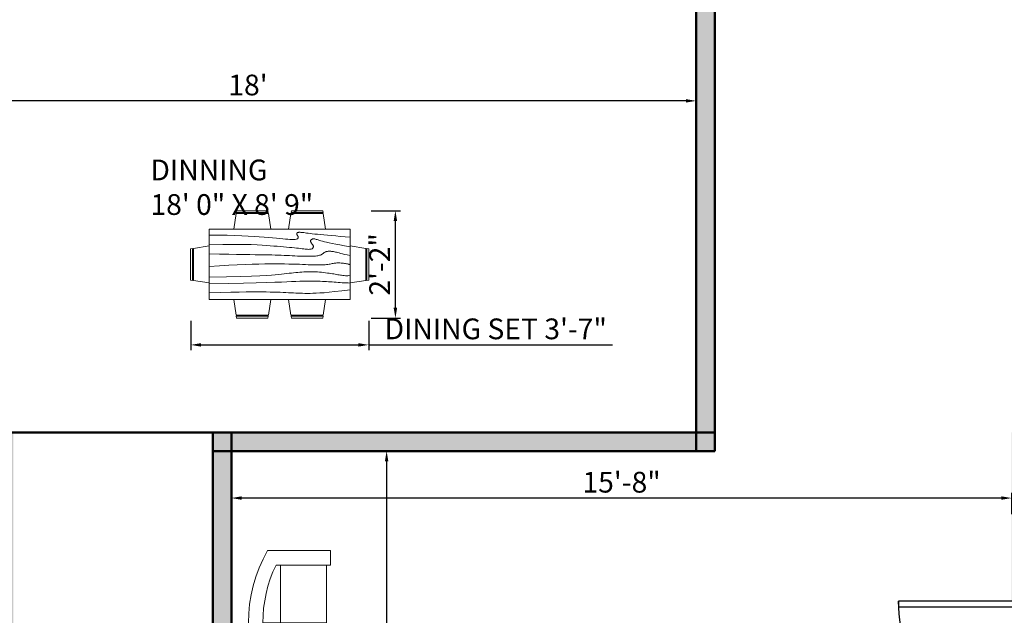
# Model space of a CAD drawing. Units: millimetres. Extents: x 3107 to 3757, y 777 to 1464.
# Tile 5 of 7: x 3301 to 3539, y 1140 to 1284. Entities that reach past the tile are written whole.
import ezdxf

# ---------------------------------------------------------------- set-up
doc = ezdxf.new("R2010")
doc.units = ezdxf.units.MM
for name, color, linetype, lineweight in [('A-ANNO-DIMS', 50, 'Continuous', 18), ('A-AREA-IDEN', 160, 'Continuous', 18), ('A-WALL-PATT', 80, 'Continuous', 13), ('doors', 10, 'Continuous', 25), ('furniture', 140, 'Continuous', 18), ('walls', 80, 'Continuous', 50)]:
    doc.layers.add(name, color=color, linetype=linetype, lineweight=lineweight)
doc.styles.get("Standard").update_dxf_attribs({"font": 'arial.ttf'})
doc.dimstyles.new('ISO-25', dxfattribs={"dimtxt": 5, "dimasz": 2.5, "dimexe": 1.25, "dimexo": 0.625, "dimtad": 1, "dimdec": 0, "dimlunit": 3, "dimtxsty": 'Standard', "dimcen": 2.5, "dimadec": 0, "dimazin": 0, "dimtfac": 1, "dimtdec": 0, "dimtmove": 0, "dimatfit": 3, "dimfxl": 1, "dimarcsym": 0})

# ---------------------------------------------------------------- blocks, each defined once
blk = doc.blocks.new('*U2')
for p, q in [((0, 0), (0, -6)), ((40, 0), (40, -6))]:
    blk.add_line(p, q)
blk.add_lwpolyline([(0, 0), (0, 40), (1.75, 40), (1.75, 0)], close=True)
blk.add_arc((0, 0), 40, 0, 90)
blk = doc.blocks.new('Dining Set - 36 x 72 in.')
for p, q in [((-22.2343, 26.00059), (-23.4847, 17.99762)), ((-22.2304, 26), (-5.7608, 26)), ((-22, 27.5), (-22.1562, 26.50042)), ((-5.8416, 26.5), (-22.1534, 26.5)), ((-22, 27.5), (-6, 27.5)), ((-5.8437, 26.49966), (-6, 27.5)), ((-4.5152, 17.99762), (-5.7655, 25.99926)), ((5.7657, 26.00059), (4.5153, 17.99762)), ((5.7696, 26), (22.2392, 26)), ((6, 27.5), (5.8438, 26.50042)), ((22.1584, 26.5), (5.8466, 26.5)), ((6, 27.5), (22, 27.5)), ((22.1563, 26.49966), (22, 27.5)), ((23.4848, 17.99762), (22.2345, 25.99926)), ((36, 18), (-36, 18)), ((-36, 18), (-36, -18)), ((36, -18), (36, 18)), ((-45.5, 8), (-44.5004, 8.15617)), ((-45.5, 8), (-45.5, -8)), ((-44.5, -8.15843), (-44.5, 8.15338)), ((-44.0006, 8.23428), (-35.9976, 9.48474)), ((-44, 8.23041), (-44, -8.23915)), ((44.0006, 8.23428), (35.9976, 9.48474)), ((44, 8.23041), (44, -8.23915)), ((44.5, -8.15843), (44.5, 8.15338)), ((45.5, 8), (44.5005, 8.15617)), ((45.5, 8), (45.5, -8)), ((-44.4997, -8.15631), (-45.5, -8)), ((-35.9976, -9.48476), (-43.9993, -8.2345)), ((35.9976, -9.48476), (43.9993, -8.2345)), ((44.4997, -8.15631), (45.5, -8)), ((-36, -18), (36, -18)), ((-22.2343, -26.0006), (-23.4847, -17.99762)), ((-4.5152, -17.99762), (-5.7655, -25.99928)), ((5.7657, -26.0006), (4.5153, -17.99762)), ((23.4848, -17.99762), (22.2345, -25.99928)), ((-22.2304, -26), (-5.7608, -26)), ((-22, -27.5), (-22.1562, -26.50044)), ((-5.8416, -26.5), (-22.1534, -26.5)), ((-22, -27.5), (-6, -27.5)), ((-5.8437, -26.49967), (-6, -27.5)), ((5.7696, -26), (22.2392, -26)), ((6, -27.5), (5.8438, -26.50044)), ((22.1584, -26.5), (5.8466, -26.5)), ((6, -27.5), (22, -27.5)), ((22.1563, -26.49967), (22, -27.5))]:
    blk.add_line(p, q)
for points in [[(-36, 15), (-31.1772, 14.97754), (-26.8079, 14.91406), (-22.8538, 14.81543), (-19.276, 14.6875), (-16.0362, 14.53613), (-13.0957, 14.36718), (-10.4159, 14.18652), (-7.9583, 14), (-5.6904, 13.81315), (-3.6035, 13.63021), (-1.6954, 13.45508), (0.0365, 13.29166), (1.5945, 13.14388), (2.9811, 13.01562), (4.1988, 12.9108), (5.25, 12.83333), (6.1393, 12.78613), (6.8802, 12.76823), (7.4883, 12.77767), (7.9792, 12.8125), (8.3685, 12.87077), (8.6719, 12.95052), (8.9049, 13.0498), (9.0833, 13.16666), (9.2205, 13.29899), (9.3216, 13.44401), (9.3895, 13.59879), (9.4271, 13.76041), (9.4373, 13.92594), (9.4232, 14.09245), (9.3875, 14.257), (9.3333, 14.41666), (9.2638, 14.56917), (9.1836, 14.71484), (9.0975, 14.85465), (9.0104, 14.98958), (8.9272, 15.1206), (8.8529, 15.2487), (8.7922, 15.37483), (8.75, 15.5), (8.7305, 15.62467), (8.7344, 15.74739), (8.7617, 15.86621), (8.8125, 15.97916), (8.8867, 16.08431), (8.9844, 16.17968), (9.1055, 16.26334), (9.25, 16.33333), (9.4189, 16.38802), (9.6172, 16.42708), (9.8506, 16.45052), (10.125, 16.45833), (10.4463, 16.45052), (10.8203, 16.42708), (11.2529, 16.38802), (11.75, 16.33333), (12.3184, 16.26318), (12.9694, 16.17838), (13.7151, 16.07991), (14.5677, 15.96875), (15.5395, 15.84586), (16.6426, 15.71224), (17.8893, 15.56884), (19.2917, 15.41666), (20.859, 15.25667), (22.5879, 15.08984), (24.4721, 14.91715), (26.5052, 14.73958), (28.6809, 14.5581), (30.9929, 14.3737), (33.4347, 14.18733), (36, 14)], [(-36, 10), (-28.9766, 10.14274), (-23.1725, 10.20442), (-18.4241, 10.19775), (-14.5677, 10.13541), (-11.4399, 10.03011), (-8.877, 9.89453), (-6.7154, 9.74137), (-4.7917, 9.58333), (-2.9698, 9.43082), (-1.2246, 9.28515), (0.4415, 9.14534), (2.026, 9.01041), (3.5266, 8.87939), (4.9408, 8.7513), (6.266, 8.62516), (7.5, 8.5), (8.6411, 8.37549), (9.6914, 8.2539), (10.6538, 8.13818), (11.5312, 8.03125), (12.3267, 7.93603), (13.043, 7.85547), (13.6831, 7.79248), (14.25, 7.75), (14.7471, 7.7303), (15.1797, 7.73307), (15.5537, 7.75732), (15.875, 7.80208), (16.1494, 7.86637), (16.3828, 7.94922), (16.5811, 8.04964), (16.75, 8.16666), (16.8944, 8.29915), (17.0143, 8.44531), (17.1089, 8.60319), (17.1771, 8.77083), (17.218, 8.94629), (17.2305, 9.1276), (17.2137, 9.31282), (17.1667, 9.5), (17.0895, 9.6875), (16.987, 9.875), (16.8649, 10.0625), (16.7292, 10.25), (16.5856, 10.4375), (16.4401, 10.625), (16.2985, 10.8125), (16.1667, 11), (16.05, 11.18733), (15.9518, 11.3737), (15.8752, 11.5581), (15.8229, 11.73958), (15.798, 11.91715), (15.8034, 12.08984), (15.842, 12.25667), (15.9167, 12.41666), (16.0295, 12.56836), (16.1784, 12.70833), (16.3605, 12.83268), (16.5729, 12.9375), (16.8127, 13.01888), (17.0768, 13.07291), (17.3625, 13.0957), (17.6667, 13.08333), (17.9894, 13.03312), (18.3418, 12.94726), (18.7382, 12.82918), (19.1927, 12.68229), (19.7195, 12.51001), (20.3327, 12.31575), (21.0465, 12.10294), (21.875, 11.875), (22.8357, 11.63354), (23.959, 11.37304), (25.2786, 11.08618), (26.8282, 10.76562), (28.6414, 10.40405), (30.752, 9.99414), (33.1936, 9.52856), (36, 9)], [(-36, 5.5), (-30.7157, 5.3348), (-26.069, 5.20963), (-21.9946, 5.11767), (-18.4271, 5.05208), (-15.3009, 5.00602), (-12.5508, 4.97265), (-10.1112, 4.94515), (-7.9167, 4.91666), (-5.909, 4.88167), (-4.0586, 4.83984), (-2.3429, 4.79215), (-0.7396, 4.73958), (0.7739, 4.6831), (2.22, 4.6237), (3.6213, 4.56233), (5, 4.5), (6.373, 4.43782), (7.7344, 4.3776), (9.0723, 4.32129), (10.375, 4.27083), (11.6309, 4.22819), (12.8281, 4.19531), (13.9551, 4.17415), (15, 4.16666), (15.954, 4.17448), (16.819, 4.19791), (17.6001, 4.23698), (18.3021, 4.29166), (18.9299, 4.36198), (19.4883, 4.44791), (19.9823, 4.54948), (20.4167, 4.66666), (20.7969, 4.79899), (21.1302, 4.94401), (21.4245, 5.09879), (21.6875, 5.26041), (21.9271, 5.42594), (22.1511, 5.59245), (22.3672, 5.757), (22.5834, 5.91666), (22.8065, 6.06868), (23.0404, 6.21093), (23.2879, 6.34147), (23.5521, 6.45833), (23.8358, 6.55957), (24.142, 6.64323), (24.4735, 6.70735), (24.8334, 6.75), (25.2235, 6.76969), (25.642, 6.76692), (26.0858, 6.74267), (26.5521, 6.69791), (27.0379, 6.63362), (27.5404, 6.55078), (28.0565, 6.45036), (28.5834, 6.33333), (29.1242, 6.19987), (29.7071, 6.04687), (30.3661, 5.87044), (31.1354, 5.66666), (32.0493, 5.43164), (33.142, 5.16146), (34.4475, 4.85221), (36, 4.5)], [(-36, -1), (-30.7915, -0.6591), (-26.0195, -0.38216), (-21.6519, -0.16284), (-17.6563, 0.00521), (-14.0005, 0.12833), (-10.6523, 0.21289), (-7.5796, 0.26522), (-4.75, 0.29166), (-2.134, 0.29793), (0.2878, 0.28711), (2.5317, 0.26163), (4.6146, 0.22396), (6.5529, 0.17651), (8.3633, 0.12174), (10.0623, 0.06209), (11.6667, 0), (13.1899, -0.06201), (14.6341, -0.1211), (15.9982, -0.17432), (17.2813, -0.21875), (18.4823, -0.25147), (19.6003, -0.26953), (20.6343, -0.27002), (21.5834, -0.25), (22.4481, -0.20768), (23.2357, -0.14584), (23.9549, -0.06836), (24.6146, 0.02083), (25.2235, 0.11784), (25.7904, 0.21875), (26.3241, 0.31966), (26.8334, 0.41666), (27.3265, 0.50618), (27.8099, 0.58593), (28.2894, 0.65397), (28.7709, 0.70833), (29.2601, 0.74707), (29.763, 0.76823), (30.2855, 0.76985), (30.8334, 0.75), (31.4088, 0.70784), (31.9994, 0.64713), (32.589, 0.57275), (33.1615, 0.48958), (33.7008, 0.4025), (34.1908, 0.3164), (34.6153, 0.23616), (34.9584, 0.16666), (35.2099, 0.11165), (35.3848, 0.07031), (35.504, 0.04069), (35.5886, 0.02083), (35.6594, 0.00879), (35.7377, 0.0026), (35.8442, 0.00032), (36, 0)], [(-36, -6.5), (-27.1843, -6.31267), (-20.084, -6.1263), (-14.469, -5.9419), (-10.1094, -5.76042), (-6.7752, -5.58285), (-4.2363, -5.41016), (-2.2629, -5.24333), (-0.625, -5.08334), (0.8708, -4.93099), (2.2715, -4.78646), (3.5872, -4.64974), (4.8281, -4.52084), (6.0046, -4.39974), (7.127, -4.28646), (8.2053, -4.18099), (9.25, -4.08334), (10.2705, -3.99382), (11.2734, -3.91407), (12.2647, -3.84603), (13.25, -3.79167), (14.2354, -3.75293), (15.2266, -3.73177), (16.2295, -3.73015), (17.25, -3.75), (18.2912, -3.79248), (19.3451, -3.85547), (20.4009, -3.93604), (21.4479, -4.03125), (22.4754, -4.13819), (23.4727, -4.25391), (24.4289, -4.37549), (25.3334, -4.5), (26.1785, -4.62492), (26.9694, -4.74935), (27.7145, -4.87281), (28.4219, -4.99479), (29.1, -5.11483), (29.7572, -5.23242), (30.4016, -5.34709), (31.0417, -5.45834), (31.6837, -5.56437), (32.3262, -5.65821), (32.9658, -5.73153), (33.599, -5.77604), (34.2224, -5.78345), (34.8327, -5.74545), (35.4264, -5.65373), (36, -5.5)], [(-36, -10), (-26.4022, -9.81299), (-18.4675, -9.62891), (-11.9839, -9.45069), (-6.7396, -9.28125), (-2.5226, -9.12354), (0.8789, -8.98047), (3.6769, -8.85498), (6.0833, -8.75), (8.2767, -8.66765), (10.3021, -8.60677), (12.1712, -8.56543), (13.8958, -8.54167), (15.4876, -8.53353), (16.9583, -8.53907), (18.3197, -8.55632), (19.5834, -8.58334), (20.7616, -8.61841), (21.8685, -8.66081), (22.9188, -8.71004), (23.9271, -8.76563), (24.9081, -8.82707), (25.8763, -8.89388), (26.8465, -8.96558), (27.8334, -9.04167), (28.8474, -9.12118), (29.8828, -9.20117), (30.93, -9.27824), (31.9792, -9.34896), (33.0205, -9.40991), (34.0443, -9.45768), (35.0407, -9.48885), (36, -9.5)], [(-36, -14.5), (-30.0881, -14.33513), (-25.0332, -14.21224), (-20.7312, -14.12647), (-17.0781, -14.07292), (-13.97, -14.04671), (-11.3027, -14.04297), (-8.9724, -14.05681), (-6.875, -14.08334), (-4.9224, -14.11833), (-3.0905, -14.16016), (-1.3709, -14.20785), (0.2448, -14.26042), (1.7647, -14.3169), (3.1973, -14.3763), (4.5507, -14.43767), (5.8333, -14.5), (7.0554, -14.5621), (8.235, -14.62175), (9.3922, -14.67652), (10.5469, -14.72396), (11.7192, -14.76164), (12.929, -14.78711), (14.1965, -14.79794), (15.5417, -14.79167), (16.9933, -14.76424), (18.6152, -14.70508), (20.4804, -14.60197), (22.6615, -14.44271), (25.2312, -14.21509), (28.2624, -13.9069), (31.8277, -13.50594), (36, -13)]]:
    blk.add_lwpolyline(points)
blk = doc.blocks.new('Sofa - Roundback Loveseat 5 ft.')
for p, q in [((0, -32.44198), (0, -5.99998)), ((-24, -33.99998), (-24, -11.46958)), ((24.00004, -33.99998), (24.00004, -11.46958)), ((-23.9998, -13.38178), (23.99986, -13.38178)), ((-24, -32.44198), (24.00004, -32.44198))]:
    blk.add_line(p, q)
for points in [[(-24, -33.99998), (-30, -33.99998), (-30, -7.99998)], [(30.00004, -7.99998), (30.00004, -33.99998), (24.00004, -33.99998)]]:
    blk.add_lwpolyline(points)
for centre, radius, start, end in [((0, -60.24998), 60.24998, 60.13715, 119.8628), ((0, -61.38438), 55.38444, 64.32083, 115.6792)]:
    blk.add_arc(centre, radius, start, end)
blk = doc.blocks.new('*D24')
at = {"layer": 'A-ANNO-DIMS', "color": 0, "lineweight": -2, "transparency": 16777216}
for p, q in [((3248.47, 1264.98), (3248.47, 1265.6)), ((3461.97, 1264.35), (3250.97, 1264.35)), ((3464.47, 1264.98), (3464.47, 1265.6))]:
    blk.add_line(p, q, dxfattribs=at)
at = {"layer": 'A-ANNO-DIMS', "color": 0, "transparency": 16777216}
for points in [[(3250.97, 1264.77), (3250.97, 1263.94), (3248.47, 1264.35)], [(3461.97, 1264.77), (3461.97, 1263.94), (3464.47, 1264.35)]]:
    blk.add_solid(points, dxfattribs=at)
at = {"layer": 'Defpoints', "color": 0, "transparency": 16777216}
for p in [(3248.47, 1264.35), (3248.47, 1264.35), (3464.47, 1264.35)]:
    blk.add_point(p, dxfattribs=at)
at = {"layer": 'A-ANNO-DIMS', "color": 0, "transparency": 16777216, "insert": (3356.47, 1267.53), "char_height": 5, "attachment_point": 5}
blk.add_mtext("18'", dxfattribs=at)
blk = doc.blocks.new('*D40')
at = {"layer": 'A-ANNO-DIMS', "color": 0, "lineweight": -2, "transparency": 16777216}
for p, q in [((3385.8, 1179.93), (3391.12, 1179.93)), ((3389.87, 1177.43), (3389.87, 1030.43)), ((3384.41, 1027.93), (3391.12, 1027.93))]:
    blk.add_line(p, q, dxfattribs=at)
at = {"layer": 'A-ANNO-DIMS', "color": 0, "transparency": 16777216}
for points in [[(3389.45, 1177.43), (3390.29, 1177.43), (3389.87, 1179.93)], [(3389.45, 1030.43), (3390.29, 1030.43), (3389.87, 1027.93)]]:
    blk.add_solid(points, dxfattribs=at)
at = {"layer": 'Defpoints', "color": 0, "transparency": 16777216}
for p in [(3385.18, 1179.93), (3383.78, 1027.93), (3389.87, 1027.93)]:
    blk.add_point(p, dxfattribs=at)
at = {"layer": 'A-ANNO-DIMS', "color": 0, "transparency": 16777216, "insert": (3386.69, 1103.93), "char_height": 5, "attachment_point": 5, "rotation": 90}
blk.add_mtext('12\'-8"', dxfattribs=at)
blk = doc.blocks.new('*D41')
at = {"layer": 'A-ANNO-DIMS', "color": 0, "lineweight": -2, "transparency": 16777216}
for p, q in [((3352.47, 1164.68), (3352.47, 1169.84)), ((3540.47, 1164.68), (3540.47, 1169.84)), ((3537.97, 1168.59), (3354.97, 1168.59))]:
    blk.add_line(p, q, dxfattribs=at)
at = {"layer": 'A-ANNO-DIMS', "color": 0, "transparency": 16777216}
for points in [[(3354.97, 1169), (3354.97, 1168.17), (3352.47, 1168.59)], [(3537.97, 1169), (3537.97, 1168.17), (3540.47, 1168.59)]]:
    blk.add_solid(points, dxfattribs=at)
at = {"layer": 'Defpoints', "color": 0, "transparency": 16777216}
for p in [(3352.47, 1168.59), (3352.47, 1164.06), (3540.47, 1164.06)]:
    blk.add_point(p, dxfattribs=at)
at = {"layer": 'A-ANNO-DIMS', "color": 0, "transparency": 16777216, "insert": (3446.47, 1171.76), "char_height": 5, "attachment_point": 5}
blk.add_mtext('15\'-8"', dxfattribs=at)
blk = doc.blocks.new('*D65')
at = {"layer": 'A-ANNO-DIMS', "color": 0, "lineweight": -2, "transparency": 16777216}
for p, q in [((3342.67, 1211.32), (3342.67, 1204.27)), ((3385.56, 1211.32), (3385.56, 1204.27)), ((3345.17, 1205.52), (3383.06, 1205.52)), ((3385.56, 1205.52), (3444.26, 1205.52))]:
    blk.add_line(p, q, dxfattribs=at)
at = {"layer": 'A-ANNO-DIMS', "color": 0, "transparency": 16777216}
for points in [[(3345.17, 1205.93), (3345.17, 1205.1), (3342.67, 1205.52)], [(3383.06, 1205.93), (3383.06, 1205.1), (3385.56, 1205.52)]]:
    blk.add_solid(points, dxfattribs=at)
at = {"layer": 'Defpoints', "color": 0, "transparency": 16777216}
for p in [(3342.67, 1211.95), (3385.56, 1211.95), (3385.56, 1205.52)]:
    blk.add_point(p, dxfattribs=at)
at = {"layer": 'A-ANNO-DIMS', "color": 0, "transparency": 16777216, "insert": (3416.16, 1208.73), "char_height": 5, "attachment_point": 5}
blk.add_mtext('DINING SET 3\'-7"', dxfattribs=at)
blk = doc.blocks.new('*D66')
at = {"layer": 'A-ANNO-DIMS', "color": 0, "lineweight": -2, "transparency": 16777216}
for p, q in [((3386.18, 1237.87), (3393.24, 1237.87)), ((3391.99, 1214.45), (3391.99, 1235.37)), ((3386.18, 1211.95), (3393.24, 1211.95))]:
    blk.add_line(p, q, dxfattribs=at)
at = {"layer": 'A-ANNO-DIMS', "color": 0, "transparency": 16777216}
for points in [[(3391.57, 1235.37), (3392.41, 1235.37), (3391.99, 1237.87)], [(3391.57, 1214.45), (3392.41, 1214.45), (3391.99, 1211.95)]]:
    blk.add_solid(points, dxfattribs=at)
at = {"layer": 'Defpoints', "color": 0, "transparency": 16777216}
for p in [(3385.56, 1237.87), (3391.99, 1237.87), (3385.56, 1211.95)]:
    blk.add_point(p, dxfattribs=at)
at = {"layer": 'A-ANNO-DIMS', "color": 0, "transparency": 16777216, "insert": (3388.85, 1224.91), "char_height": 5, "attachment_point": 5, "rotation": 90}
blk.add_mtext('2\'-2"', dxfattribs=at)

msp = doc.modelspace()

# ---------------------------------------------------------------- hatches: boundary and pattern name
at = {"layer": 'A-WALL-PATT'}
h = msp.add_hatch(color=256, dxfattribs=at)
h.dxf.hatch_style = 1
h.paths.add_polyline_path([(3119.47, 1087.39), (3110.47, 1087.39), (3110.47, 1027.93), (3119.47, 1027.93)])
h.paths.add_polyline_path([(3119.47, 1027.93), (3110.47, 1027.93), (3110.47, 1023.43), (3119.47, 1023.43)])
h.paths.add_polyline_path([(3267.47, 1027.93), (3119.47, 1027.93), (3119.47, 1023.43), (3267.47, 1023.43)])
h.paths.add_polyline_path([(3119.47, 1023.43), (3110.47, 1023.43), (3110.47, 979.44), (3119.47, 979.44)])
h.paths.add_polyline_path([(3299.97, 1179.93), (3295.47, 1179.93), (3295.47, 1027.93), (3299.97, 1027.93)])
h.paths.add_polyline_path([(3295.47, 1027.93), (3271.97, 1027.93), (3271.97, 1023.43), (3295.47, 1023.43)])
h.paths.add_polyline_path([(3271.97, 1027.93), (3267.47, 1027.93), (3267.47, 1023.43), (3271.97, 1023.43)])
h.paths.add_polyline_path([(3299.97, 1027.93), (3295.47, 1027.93), (3295.47, 1023.43), (3299.97, 1023.43)])
h.paths.add_polyline_path([(3299.97, 1184.43), (3295.47, 1184.43), (3295.47, 1179.93), (3299.97, 1179.93)])
h.paths.add_polyline_path([(3295.47, 1184.43), (3288.38, 1184.43), (3288.38, 1182.47), (3288.38, 1179.93), (3295.47, 1179.93)])
h.paths.add_polyline_path([(3352.47, 1179.93), (3347.97, 1179.93), (3347.97, 1027.93), (3352.47, 1027.93)])
h.paths.add_polyline_path([(3352.47, 1184.43), (3347.97, 1184.43), (3347.97, 1179.93), (3352.47, 1179.93)])
h.paths.add_polyline_path([(3464.47, 1184.43), (3352.47, 1184.43), (3352.47, 1179.93), (3464.47, 1179.93)])
h.paths.add_polyline_path([(3468.97, 1288.93), (3464.47, 1288.93), (3464.47, 1184.43), (3468.97, 1184.43)])
h.paths.add_polyline_path([(3468.97, 1184.43), (3464.47, 1184.43), (3464.47, 1179.93), (3468.97, 1179.93)])
h.paths.add_polyline_path([(3195.97, 1248.43), (3191.47, 1248.43), (3191.47, 1184.43), (3195.97, 1184.43)])
h.paths.add_polyline_path([(3195.97, 1184.43), (3191.47, 1184.43), (3191.47, 1179.93), (3195.97, 1179.93)])
h.paths.add_polyline_path([(3191.47, 1184.43), (3183.28, 1184.43), (3183.28, 1181.58), (3183.28, 1179.93), (3191.47, 1179.93)])
h.paths.add_polyline_path([(3243.97, 1184.43), (3195.97, 1184.43), (3195.97, 1179.93), (3243.97, 1179.93)])
h.paths.add_polyline_path([(3257.91, 1182.47), (3257.91, 1184.43), (3248.47, 1184.43), (3248.47, 1179.93), (3258.02, 1179.93, -0.020891)])
h.paths.add_polyline_path([(3248.47, 1184.43), (3243.97, 1184.43), (3243.97, 1179.93), (3248.47, 1179.93)])
h.paths.add_polyline_path([(3248.47, 1189.24), (3247.51, 1189.24), (3243.97, 1189.24), (3243.97, 1184.43), (3248.47, 1184.43)])
h.paths.add_polyline_path([(3166.87, 1184.43), (3119.47, 1184.43), (3119.47, 1179.93), (3166.63, 1179.93), (3166.63, 1181.58, -0.042981)])
h.paths.add_polyline_path([(3119.47, 1184.43), (3110.47, 1184.43), (3110.47, 1179.93), (3119.47, 1179.93)])
h.paths.add_polyline_path([(3119.47, 1248.43), (3110.47, 1248.43), (3110.47, 1184.43), (3119.47, 1184.43)])
h.paths.add_polyline_path([(3119.47, 1179.93), (3110.47, 1179.93), (3110.47, 1140.65), (3119.47, 1140.65)])
h.paths.add_polyline_path([(3119.47, 1288.93), (3110.47, 1288.93), (3110.47, 1252.93), (3119.47, 1252.93)])
h.paths.add_polyline_path([(3119.47, 1252.93), (3110.47, 1252.93), (3110.47, 1248.43), (3119.47, 1248.43)])
h.paths.add_polyline_path([(3191.47, 1252.93), (3119.47, 1252.93), (3119.47, 1248.43), (3191.47, 1248.43)])
h.paths.add_polyline_path([(3195.97, 1288.93), (3191.47, 1288.93), (3191.47, 1252.93), (3195.97, 1252.93)])
h.paths.add_polyline_path([(3195.97, 1252.93), (3191.47, 1252.93), (3191.47, 1248.43), (3195.97, 1248.43)])
h.paths.add_polyline_path([(3248.47, 1293.43), (3243.97, 1293.43), (3243.97, 1288.93), (3248.47, 1288.93)])
h.paths.add_polyline_path([(3243.97, 1293.43), (3195.97, 1293.43), (3195.97, 1288.93), (3243.97, 1288.93)])
h.paths.add_polyline_path([(3303.47, 1293.43), (3248.47, 1293.43), (3248.47, 1288.93), (3303.47, 1288.93)])
h.paths.add_polyline_path([(3248.47, 1288.93), (3243.97, 1288.93), (3243.97, 1205.51, -0.053712), (3247.51, 1205.89), (3248.47, 1205.89)])
h.paths.add_polyline_path([(3191.47, 1293.43), (3119.47, 1293.43), (3119.47, 1288.93), (3191.47, 1288.93)])
h.paths.add_polyline_path([(3119.47, 1293.43), (3110.47, 1293.43), (3110.47, 1288.93), (3119.47, 1288.93)])
h.paths.add_polyline_path([(3119.47, 1322.96, -0.065064), (3111.64, 1321.93), (3110.47, 1321.93), (3110.47, 1293.43), (3119.47, 1293.43)])
h.paths.add_polyline_path([(3195.97, 1293.43), (3191.47, 1293.43), (3191.47, 1288.93), (3195.97, 1288.93)])
h.paths.add_polyline_path([(3119.47, 1450.43), (3110.47, 1450.43), (3110.47, 1441.43), (3119.47, 1441.43)])
h.paths.add_polyline_path([(3119.47, 1441.43), (3110.47, 1441.43), (3110.47, 1352.4), (3111.64, 1352.4), (3119.47, 1352.4)])
h.paths.add_polyline_path([(3176.58, 1450.43), (3119.47, 1450.43), (3119.47, 1441.43), (3176.58, 1441.43)])
h.paths.add_polyline_path([(3323.19, 1450.43), (3307.97, 1450.43), (3307.97, 1441.43), (3323.19, 1441.43)])
h.paths.add_polyline_path([(3307.97, 1450.43), (3303.47, 1450.43), (3303.47, 1441.43), (3307.97, 1441.43)])
h.paths.add_polyline_path([(3303.47, 1450.43), (3229.4, 1450.43), (3229.4, 1441.43), (3303.47, 1441.43)])
h.paths.add_polyline_path([(3307.97, 1441.43), (3303.47, 1441.43), (3303.47, 1363.43), (3307.97, 1363.43)])
h.paths.add_polyline_path([(3307.97, 1363.43), (3303.47, 1363.43), (3303.47, 1358.93), (3307.97, 1358.93)])
h.paths.add_polyline_path([(3307.97, 1358.93), (3303.47, 1358.93), (3303.47, 1342.3), (3305.5, 1342.3, -0.037178), (3307.97, 1342.12)])
h.paths.add_polyline_path([(3379.97, 1363.43), (3307.97, 1363.43), (3307.97, 1358.93), (3379.97, 1358.93)])
h.paths.add_polyline_path([(3384.47, 1393.61), (3383.04, 1393.61), (3379.97, 1393.61), (3379.97, 1363.43), (3384.47, 1363.43)])
h.paths.add_polyline_path([(3384.47, 1363.43), (3379.97, 1363.43), (3379.97, 1358.93), (3384.47, 1358.93)])
h.paths.add_polyline_path([(3384.47, 1358.93), (3379.97, 1358.93), (3379.97, 1293.43), (3384.47, 1293.43)])
h.paths.add_polyline_path([(3384.47, 1441.43), (3379.97, 1441.43), (3379.97, 1409.98, -0.046389), (3383.04, 1410.27), (3384.47, 1410.27)])
h.paths.add_polyline_path([(3384.47, 1450.43), (3379.97, 1450.43), (3379.97, 1441.43), (3384.47, 1441.43)])
h.paths.add_polyline_path([(3379.97, 1450.43), (3357.18, 1450.43), (3357.18, 1441.43), (3379.97, 1441.43)])
h.paths.add_polyline_path([(3432.79, 1450.43), (3384.47, 1450.43), (3384.47, 1441.43), (3432.79, 1441.43)])
h.paths.add_polyline_path([(3540.47, 1450.43), (3484.18, 1450.43), (3484.18, 1441.43), (3540.47, 1441.43)])
h.paths.add_polyline_path([(3544.97, 1450.43), (3540.47, 1450.43), (3540.47, 1441.43), (3544.97, 1441.43)])
h.paths.add_polyline_path([(3544.97, 1441.43), (3540.47, 1441.43), (3540.47, 1293.43), (3544.97, 1293.43)])
h.paths.add_polyline_path([(3590.83, 1450.43), (3544.97, 1450.43), (3544.97, 1441.43), (3590.83, 1441.43)])
h.paths.add_polyline_path([(3712.97, 1450.43), (3645.62, 1450.43), (3645.62, 1441.43), (3712.97, 1441.43)])
h.paths.add_polyline_path([(3721.97, 1441.43), (3712.97, 1441.43), (3712.97, 1288.93), (3712.97, 1184.43), (3721.97, 1184.43), (3721.97, 1288.93)])
h.paths.add_polyline_path([(3721.97, 1450.43), (3712.97, 1450.43), (3712.97, 1441.43), (3721.97, 1441.43)])
h.paths.add_polyline_path([(3712.97, 1184.43), (3658.24, 1184.43), (3658.24, 1183.15), (3658.24, 1179.93), (3712.97, 1179.93)])
h.paths.add_polyline_path([(3721.97, 1184.43), (3712.97, 1184.43), (3712.97, 1179.93), (3721.97, 1179.93)])
h.paths.add_polyline_path([(3597.32, 1183.15), (3597.32, 1184.43), (3544.97, 1184.43), (3544.97, 1179.93), (3597.32, 1179.93)])
h.paths.add_polyline_path([(3544.97, 1184.43), (3540.47, 1184.43), (3540.47, 1179.93), (3544.97, 1179.93)])
h.paths.add_polyline_path([(3544.97, 1179.93), (3540.47, 1179.93), (3540.47, 1143.69), (3543.65, 1143.69), (3544.97, 1143.69)])
h.paths.add_polyline_path([(3721.97, 1179.93), (3712.97, 1179.93), (3712.97, 1006.22), (3712.97, 871.43), (3721.97, 871.43), (3721.97, 1006.22)])
h.paths.add_polyline_path([(3468.97, 1293.43), (3464.47, 1293.43), (3464.47, 1288.93), (3468.97, 1288.93)])
h.paths.add_polyline_path([(3540.47, 1293.43), (3468.97, 1293.43), (3468.97, 1288.93), (3540.47, 1288.93)])
h.paths.add_polyline_path([(3544.97, 1293.43), (3540.47, 1293.43), (3540.47, 1288.93), (3544.97, 1288.93)])
h.paths.add_polyline_path([(3464.47, 1293.43), (3417.83, 1293.43, -0.015057), (3417.88, 1291.6), (3417.88, 1288.93), (3464.47, 1288.93)])
h.paths.add_polyline_path([(3379.97, 1293.43), (3307.97, 1293.43), (3307.97, 1288.93), (3379.97, 1288.93)])
h.paths.add_polyline_path([(3307.97, 1325.65), (3305.5, 1325.65), (3303.47, 1325.65), (3303.47, 1293.43), (3307.97, 1293.43)])
h.paths.add_polyline_path([(3307.97, 1293.43), (3303.47, 1293.43), (3303.47, 1288.93), (3307.97, 1288.93)])
h.paths.add_polyline_path([(3384.47, 1293.43), (3379.97, 1293.43), (3379.97, 1288.93), (3384.47, 1288.93)])
h.paths.add_polyline_path([(3387.42, 1291.6), (3387.42, 1293.43), (3384.47, 1293.43), (3384.47, 1288.93), (3387.42, 1288.93)])
h.paths.add_polyline_path([(3119.47, 927.28), (3110.47, 927.28), (3110.47, 871.43), (3119.47, 871.43)])
h.paths.add_polyline_path([(3119.47, 871.43), (3110.47, 871.43), (3110.47, 862.43), (3119.47, 862.43)])
h.paths.add_polyline_path([(3267.47, 871.43), (3119.47, 871.43), (3119.47, 862.43), (3267.47, 862.43)])
h.paths.add_polyline_path([(3271.97, 971.43), (3267.47, 971.43), (3267.47, 871.43), (3271.97, 871.43)])
h.paths.add_polyline_path([(3271.97, 871.43), (3267.47, 871.43), (3267.47, 862.43), (3271.97, 862.43)])
h.paths.add_polyline_path([(3287.13, 871.43), (3271.97, 871.43), (3271.97, 862.43), (3287.13, 862.43)])
h.paths.add_polyline_path([(3347.97, 871.43), (3318.96, 871.43), (3318.96, 862.43), (3347.97, 862.43)])
h.paths.add_polyline_path([(3352.47, 971.43), (3347.97, 971.43), (3347.97, 871.43), (3352.47, 871.43)])
h.paths.add_polyline_path([(3352.47, 871.43), (3347.97, 871.43), (3347.97, 862.43), (3352.47, 862.43)])
h.paths.add_polyline_path([(3375.96, 871.43), (3352.47, 871.43), (3352.47, 862.43), (3375.96, 862.43)])
h.paths.add_polyline_path([(3352.47, 975.93), (3347.97, 975.93), (3347.97, 971.43), (3352.47, 971.43)])
h.paths.add_polyline_path([(3352.47, 986.27, -0.01722), (3350.37, 986.2), (3347.97, 986.2), (3347.97, 975.93), (3352.47, 975.93)])
h.paths.add_polyline_path([(3347.97, 975.93), (3292.38, 975.93), (3292.38, 973.47, -0.030785), (3292.25, 971.43), (3347.97, 971.43)])
h.paths.add_polyline_path([(3271.97, 985.98), (3269.95, 985.98), (3267.47, 985.98), (3267.47, 975.93), (3271.97, 975.93)])
h.paths.add_polyline_path([(3271.97, 975.93), (3267.47, 975.93), (3267.47, 971.43), (3271.97, 971.43)])
h.paths.add_polyline_path([(3275.72, 975.93), (3271.97, 975.93), (3271.97, 971.43), (3275.72, 971.43), (3275.72, 973.47)])
h.paths.add_polyline_path([(3271.97, 1023.43), (3267.47, 1023.43), (3267.47, 1016.34, -0.020418), (3269.95, 1016.44), (3271.97, 1016.44)])
h.paths.add_polyline_path([(3352.47, 1023.43), (3347.97, 1023.43), (3347.97, 1016.67), (3350.37, 1016.67), (3352.47, 1016.67)])
h.paths.add_polyline_path([(3352.47, 1027.93), (3347.97, 1027.93), (3347.97, 1023.43), (3352.47, 1023.43)])
h.paths.add_polyline_path([(3476.47, 1027.93), (3352.47, 1027.93), (3352.47, 1023.43), (3476.47, 1023.43)])
h.paths.add_polyline_path([(3540.47, 1027.93), (3480.97, 1027.93), (3480.97, 1023.43), (3540.47, 1023.43)])
h.paths.add_polyline_path([(3480.97, 1027.93), (3476.47, 1027.93), (3476.47, 1023.43), (3480.97, 1023.43)])
h.paths.add_polyline_path([(3480.97, 1023.43), (3476.47, 1023.43), (3476.47, 871.43), (3480.97, 871.43)])
h.paths.add_polyline_path([(3476.47, 871.43), (3429.88, 871.43), (3429.88, 862.43), (3476.47, 862.43)])
h.paths.add_polyline_path([(3480.97, 871.43), (3476.47, 871.43), (3476.47, 862.43), (3480.97, 862.43)])
h.paths.add_polyline_path([(3493.81, 871.43), (3480.97, 871.43), (3480.97, 862.43), (3493.81, 862.43)])
h.paths.add_polyline_path([(3712.97, 871.43), (3525.61, 871.43), (3525.61, 862.43), (3712.97, 862.43)])
h.paths.add_polyline_path([(3721.97, 871.43), (3712.97, 871.43), (3712.97, 862.43), (3721.97, 862.43)])

# ---------------------------------------------------------------- linework, layer by layer
at = {"layer": 'walls'}
for p, q in [((3464.47, 1293.43), (3464.47, 1179.93)), ((3468.97, 1293.43), (3468.97, 1179.93)), ((3288.38, 1184.43), (3468.97, 1184.43)), ((3347.97, 1184.43), (3347.97, 1016.67)), ((3352.47, 1184.43), (3352.47, 1016.67)), ((3347.97, 1179.93), (3468.97, 1179.93))]:
    msp.add_line(p, q, dxfattribs=at)

# ---------------------------------------------------------------- block references
at = {"layer": 'doors', "xscale": -0.7615706373352984, "yscale": 0.7615706373352984, "zscale": 0.7615706373352984, "rotation": 90.00000000000007}
msp.add_blockref('*U2', (3543.65, 1143.69), dxfattribs=at)
at = {"layer": 'furniture', "xscale": 0.471293609702731, "yscale": 0.471293609702731, "zscale": 0.471293609702731}
msp.add_blockref('Dining Set - 36 x 72 in.', (3364.11, 1224.91), dxfattribs=at)
at = {"layer": 'furniture', "xscale": 0.5809767439628069, "yscale": 0.5809767439628069, "zscale": 0.5809767439628069, "rotation": 89.99996919953323}
msp.add_blockref('Sofa - Roundback Loveseat 5 ft.', (3356.57, 1138.5), dxfattribs=at)

# ---------------------------------------------------------------- texts
at = {"layer": 'A-AREA-IDEN', "insert": (3332.98, 1250.19), "char_height": 5, "attachment_point": 1}
msp.add_mtext_dynamic_manual_height_columns('DINNING\\P18\' 0" X 8\' 9"', width=53.6366, gutter_width=12.5, heights=[0], dxfattribs=at)

# ---------------------------------------------------------------- dimensions: what is measured, and where the dimension line sits
at = {"layer": 'A-ANNO-DIMS'}
for base, p1, p2, picture, middle in [((3248.47, 1264.35), (3464.47, 1264.35), (3248.47, 1264.35), '*D24', (3356.47, 1267.53)), ((3352.47, 1168.59), (3540.47, 1164.06), (3352.47, 1164.06), '*D41', (3446.47, 1171.76))]:
    dim = msp.add_linear_dim(base=base, p1=p1, p2=p2, dimstyle='ISO-25', override={"dimclrd": 0, "dimclre": 0, "dimclrt": 0}, dxfattribs=at)
    dim.commit()
    dim.dimension.update_dxf_attribs({"geometry": picture, "text_midpoint": middle})
for base, p1, p2, override, picture, middle in [((3391.99, 1237.87), (3385.56, 1211.95), (3385.56, 1237.87), {"dimdec": 1, "dimlfac": 1, "dimrnd": 0, "dimzin": 1, "dimdsep": 46, "dimlunit": 4, "dimfrac": 2}, '*D66', (3388.85, 1224.91)), ((3389.87, 1027.93), (3385.18, 1179.93), (3383.78, 1027.93), {"dimclrd": 0, "dimclre": 0, "dimclrt": 0}, '*D40', (3386.69, 1103.93))]:
    dim = msp.add_linear_dim(base=base, p1=p1, p2=p2, angle=90, dimstyle='ISO-25', override=override, dxfattribs=at)
    dim.commit()
    dim.dimension.update_dxf_attribs({"geometry": picture, "text_midpoint": middle})
dim = msp.add_linear_dim(base=(3385.56, 1205.52), p1=(3342.67, 1211.95), p2=(3385.56, 1211.95), text='DINING SET <>', dimstyle='ISO-25', override={"dimdec": 1, "dimlfac": 1, "dimrnd": 0, "dimzin": 1, "dimdsep": 46, "dimlunit": 4, "dimfrac": 2}, dxfattribs=at)
dim.commit()
dim.dimension.update_dxf_attribs({"geometry": '*D65', "text_midpoint": (3416.16, 1208.73)})

doc.saveas('drawing.dxf')
